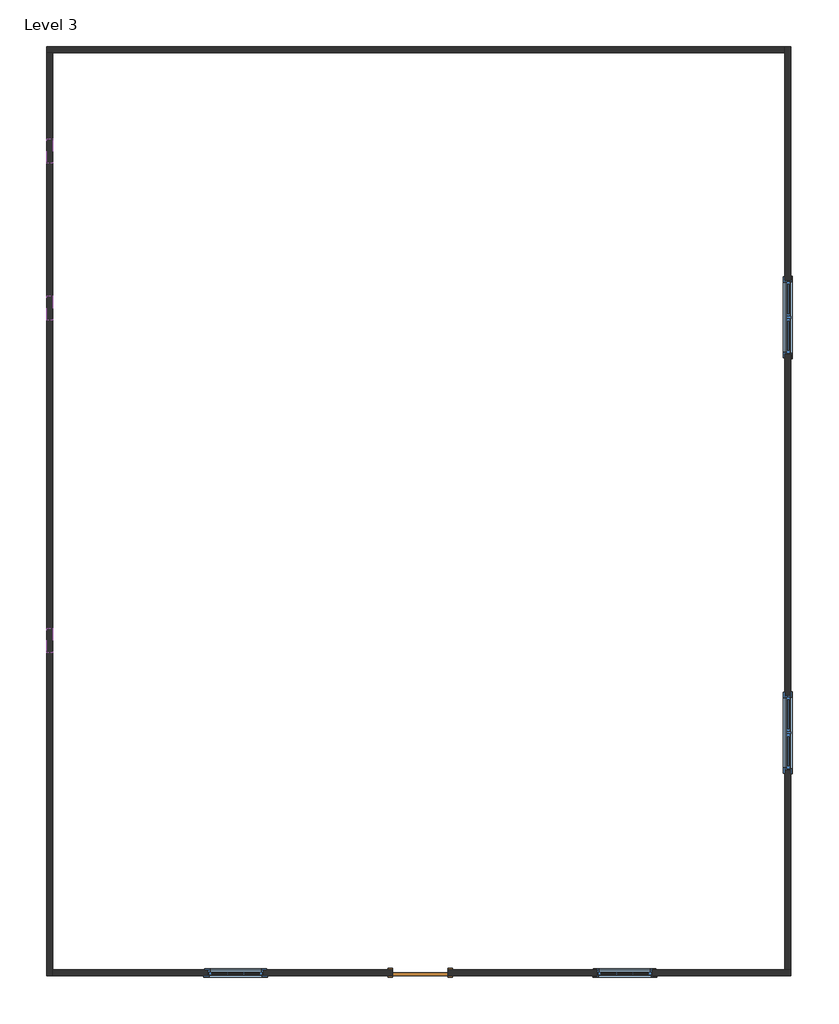
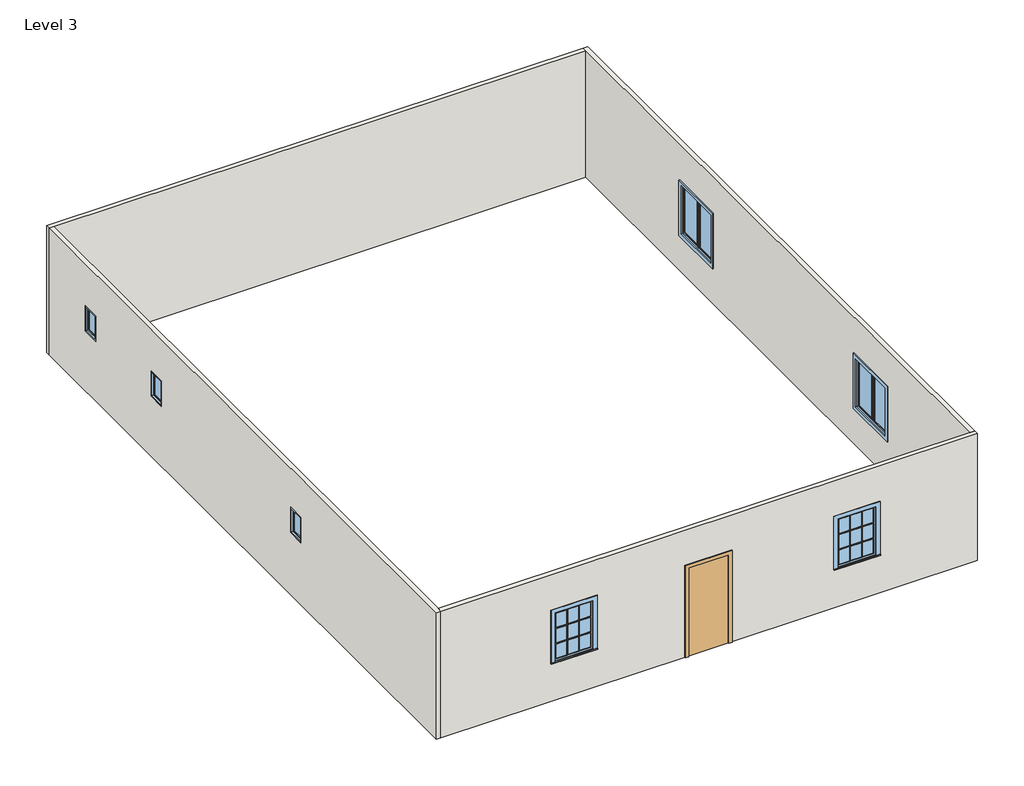
# One storey, incomplete: 7 windows, 4 walls, 1 door.
"""IFC4 building model written with IfcOpenShell, lengths in millimetres."""

from ifc_helpers import new_model, si_unit, origin, place, context, project, spatial, faceted_brep, transform, mapped, element, save
from components import door_048588e9, window_ad8769eb, window_90ef9153, window_a112695e

model = new_model("IFC4")

# Units and contexts
model_context = context("Model", 3, world=origin())
ifc_project = project(units=[si_unit("LENGTHUNIT", "METRE", prefix="MILLI")], contexts=[model_context])

# Site, building, storey
site = spatial("IfcSite", under=ifc_project)
building = spatial("IfcBuilding", under=site)
storey = spatial("IfcBuildingStorey", under=building, Name="Level 3", Elevation=3200.4)

# Door
placement = place(None, origin())
door_shape = door_048588e9(model_context)
element("IfcDoor", 1, ObjectType="Single-Flush : 36\" x 84\"", at=placement, inside=storey, context=model_context, shape_type="MappedRepresentation", body=[
    mapped(door_shape, transform((7865.9168112, -1990.8718204, 3200.4), x_axis=(-1.0, 0.0, 0.0), y_axis=(0.0, -1.0, 0.0), z_axis=(0.0, 0.0, 1.0))),
])

# Walls
element("IfcWall", 2, ObjectType="Generic - 4\" Brick", at=placement, inside=storey, context=model_context, shape_type="Brep", body=[
    faceted_brep([(1693.7168112, 13198.3281796, 3200.4), (1795.3168112, 13198.3281796, 3200.4), (13885.7168112, 13198.3281796, 3200.4), (13885.7168112, 13198.3281796, 6248.4), (1795.3168112, 13198.3281796, 6248.4), (1693.7168112, 13198.3281796, 6248.4), (1693.7168112, 13299.9281796, 3200.4), (1693.7168112, 13299.9281796, 6248.4), (13885.7168112, 13299.9281796, 6248.4), (13885.7168112, 13299.9281796, 3200.4)], [[[0, 1, 2, 3, 4, 5]], [[6, 7, 8, 9]], [[2, 1, 0, 6, 9]], [[0, 5, 7, 6]], [[3, 2, 9, 8]], [[5, 4, 3, 8, 7]]]),
])
element("IfcWall", 3, ObjectType="Generic - 4\" Brick", at=placement, inside=storey, context=model_context, shape_type="Brep", body=[
    faceted_brep([(1795.3168112, -2041.6718204, 3200.4), (1795.3168112, -1940.0718204, 3200.4), (1795.3168112, 13198.3281796, 3200.4), (1795.3168112, 13198.3281796, 6248.4), (1795.3168112, -1940.0718204, 6248.4), (1795.3168112, -2041.6718204, 6248.4), (1795.3168112, 8778.7281796, 5251.7031181), (1795.3168112, 9185.1281796, 5251.7031181), (1795.3168112, 9185.1281796, 4642.1031181), (1795.3168112, 8778.7281796, 4642.1031181), (1795.3168112, 11369.5281796, 5244.8693959), (1795.3168112, 11775.9281796, 5244.8693959), (1795.3168112, 11775.9281796, 4635.2693959), (1795.3168112, 11369.5281796, 4635.2693959), (1795.3168112, 3292.3281796, 5302.8886462), (1795.3168112, 3698.7281796, 5302.8886462), (1795.3168112, 3698.7281796, 4693.2886462), (1795.3168112, 3292.3281796, 4693.2886462), (1693.7168112, -2041.6718204, 3200.4), (1693.7168112, -2041.6718204, 6248.4), (1693.7168112, 13198.3281796, 6248.4), (1693.7168112, 13198.3281796, 3200.4), (1693.7168112, 8778.7281796, 5251.7031181), (1693.7168112, 8778.7281796, 4642.1031181), (1693.7168112, 9185.1281796, 4642.1031181), (1693.7168112, 9185.1281796, 5251.7031181), (1693.7168112, 11369.5281796, 5244.8693959), (1693.7168112, 11369.5281796, 4635.2693959), (1693.7168112, 11775.9281796, 4635.2693959), (1693.7168112, 11775.9281796, 5244.8693959), (1693.7168112, 3292.3281796, 5302.8886462), (1693.7168112, 3292.3281796, 4693.2886462), (1693.7168112, 3698.7281796, 4693.2886462), (1693.7168112, 3698.7281796, 5302.8886462)], [[[0, 1, 2, 3, 4, 5], [6, 7, 8, 9], [10, 11, 12, 13], [14, 15, 16, 17]], [[18, 19, 20, 21], [22, 23, 24, 25], [26, 27, 28, 29], [30, 31, 32, 33]], [[2, 1, 0, 18, 21]], [[0, 5, 19, 18]], [[3, 2, 21, 20]], [[5, 4, 3, 20, 19]], [[23, 22, 6, 9]], [[24, 23, 9, 8]], [[25, 24, 8, 7]], [[22, 25, 7, 6]], [[27, 26, 10, 13]], [[28, 27, 13, 12]], [[29, 28, 12, 11]], [[26, 29, 11, 10]], [[31, 30, 14, 17]], [[32, 31, 17, 16]], [[33, 32, 16, 15]], [[30, 33, 15, 14]]]),
])
element("IfcWall", 4, ObjectType="Generic - 4\" Brick", at=placement, inside=storey, context=model_context, shape_type="Brep", body=[
    faceted_brep([(7408.7168112, -1940.0718204, 5334.0), (7408.7168112, -1940.0718204, 3200.4), (1795.3168112, -1940.0718204, 3200.4), (1795.3168112, -1940.0718204, 6248.4), (13885.7168112, -1940.0718204, 6248.4), (13987.3168112, -1940.0718204, 6248.4), (13987.3168112, -1940.0718204, 3200.4), (13885.7168112, -1940.0718204, 3200.4), (8323.1168112, -1940.0718204, 3200.4), (8323.1168112, -1940.0718204, 5334.0), (4360.7168112, -1940.0718204, 5326.8905427), (4360.7168112, -1940.0718204, 4107.6905427), (5275.1168112, -1940.0718204, 4107.6905427), (5275.1168112, -1940.0718204, 5326.8905427), (10786.9168112, -1940.0718204, 5334.0), (10786.9168112, -1940.0718204, 4114.8), (11701.3168112, -1940.0718204, 4114.8), (11701.3168112, -1940.0718204, 5334.0), (1795.3168112, -2041.6718204, 3200.4), (7408.7168112, -2041.6718204, 3200.4), (7408.7168112, -2041.6718204, 5334.0), (8323.1168112, -2041.6718204, 5334.0), (8323.1168112, -2041.6718204, 3200.4), (13987.3168112, -2041.6718204, 3200.4), (13987.3168112, -2041.6718204, 6248.4), (1795.3168112, -2041.6718204, 6248.4), (4360.7168112, -2041.6718204, 5326.8905427), (5275.1168112, -2041.6718204, 5326.8905427), (5275.1168112, -2041.6718204, 4107.6905427), (4360.7168112, -2041.6718204, 4107.6905427), (10786.9168112, -2041.6718204, 5334.0), (11701.3168112, -2041.6718204, 5334.0), (11701.3168112, -2041.6718204, 4114.8), (10786.9168112, -2041.6718204, 4114.8)], [[[0, 1, 2, 3, 4, 5, 6, 7, 8, 9], [10, 11, 12, 13], [14, 15, 16, 17]], [[18, 19, 20, 21, 22, 23, 24, 25], [26, 27, 28, 29], [30, 31, 32, 33]], [[2, 1, 19, 18]], [[8, 7, 6, 23, 22]], [[6, 5, 24, 23]], [[3, 2, 18, 25]], [[5, 4, 3, 25, 24]], [[20, 19, 1, 0]], [[21, 20, 0, 9]], [[22, 21, 9, 8]], [[11, 10, 26, 29]], [[12, 11, 29, 28]], [[13, 12, 28, 27]], [[10, 13, 27, 26]], [[15, 14, 30, 33]], [[16, 15, 33, 32]], [[17, 16, 32, 31]], [[14, 17, 31, 30]]]),
])
element("IfcWall", 5, ObjectType="Generic - 4\" Brick", at=placement, inside=storey, context=model_context, shape_type="Brep", body=[
    faceted_brep([(13885.7168112, 13299.9281796, 3200.4), (13885.7168112, 13198.3281796, 3200.4), (13885.7168112, -1940.0718204, 3200.4), (13885.7168112, -1940.0718204, 6248.4), (13885.7168112, 13198.3281796, 6248.4), (13885.7168112, 13299.9281796, 6248.4), (13885.7168112, 1361.9281796, 5334.0), (13885.7168112, 1361.9281796, 4114.8), (13885.7168112, 2581.1281796, 4114.8), (13885.7168112, 2581.1281796, 5334.0), (13885.7168112, 8219.9281796, 5334.0), (13885.7168112, 8219.9281796, 4114.8), (13885.7168112, 9439.1281796, 4114.8), (13885.7168112, 9439.1281796, 5334.0), (13987.3168112, 13299.9281796, 3200.4), (13987.3168112, 13299.9281796, 6248.4), (13987.3168112, -1940.0718204, 6248.4), (13987.3168112, -1940.0718204, 3200.4), (13987.3168112, 1361.9281796, 5334.0), (13987.3168112, 2581.1281796, 5334.0), (13987.3168112, 2581.1281796, 4114.8), (13987.3168112, 1361.9281796, 4114.8), (13987.3168112, 8219.9281796, 5334.0), (13987.3168112, 9439.1281796, 5334.0), (13987.3168112, 9439.1281796, 4114.8), (13987.3168112, 8219.9281796, 4114.8)], [[[0, 1, 2, 3, 4, 5], [6, 7, 8, 9], [10, 11, 12, 13]], [[14, 15, 16, 17], [18, 19, 20, 21], [22, 23, 24, 25]], [[2, 1, 0, 14, 17]], [[0, 5, 15, 14]], [[3, 2, 17, 16]], [[5, 4, 3, 16, 15]], [[7, 6, 18, 21]], [[8, 7, 21, 20]], [[9, 8, 20, 19]], [[6, 9, 19, 18]], [[11, 10, 22, 25]], [[12, 11, 25, 24]], [[13, 12, 24, 23]], [[10, 13, 23, 22]]]),
])

# Windows
window_shape = window_ad8769eb(model_context)
element("IfcWindow", 6, ObjectType="Casement 3x3 with Trim : 36\" x 48\"", at=placement, inside=storey, context=model_context, shape_type="MappedRepresentation", body=[
    mapped(window_shape, transform((4817.9168112, -1990.8718204, 3193.2905427), x_axis=(-1.0, 0.0, 0.0), y_axis=(0.0, -1.0, 0.0), z_axis=(0.0, 0.0, 1.0))),
])
element("IfcWindow", 7, ObjectType="Casement 3x3 with Trim : 36\" x 48\"", at=placement, inside=storey, context=model_context, shape_type="MappedRepresentation", body=[
    mapped(window_shape, transform((11244.1168112, -1990.8718204, 3200.4), x_axis=(-1.0, 0.0, 0.0), y_axis=(0.0, -1.0, 0.0), z_axis=(0.0, 0.0, 1.0))),
])
window_2_shape = window_90ef9153(model_context)
element("IfcWindow", 8, ObjectType="Casement Dbl with Trim : 48\" x 48\"", at=placement, inside=storey, context=model_context, shape_type="MappedRepresentation", body=[
    mapped(window_2_shape, transform((13917.4668112, 1971.5281796, 3200.4), x_axis=(0.0, -1.0, 0.0), y_axis=(1.0, 0.0, 0.0), z_axis=(0.0, 0.0, 1.0))),
])
element("IfcWindow", 9, ObjectType="Casement Dbl with Trim : 48\" x 48\"", at=placement, inside=storey, context=model_context, shape_type="MappedRepresentation", body=[
    mapped(window_2_shape, transform((13917.4668112, 8829.5281796, 3200.4), x_axis=(0.0, -1.0, 0.0), y_axis=(1.0, 0.0, 0.0), z_axis=(0.0, 0.0, 1.0))),
])
window_3_shape = window_a112695e(model_context)
element("IfcWindow", 10, ObjectType="Fixed : 16\" x 24\"", at=placement, inside=storey, context=model_context, shape_type="MappedRepresentation", body=[
    mapped(window_3_shape, transform((1744.5168112, 8943.8281796, 3727.7031181), x_axis=(0.0, -1.0, 0.0), y_axis=(1.0, 0.0, 0.0), z_axis=(0.0, 0.0, 1.0))),
])
element("IfcWindow", 11, ObjectType="Fixed : 16\" x 24\"", at=placement, inside=storey, context=model_context, shape_type="MappedRepresentation", body=[
    mapped(window_3_shape, transform((1744.5168112, 11534.6281796, 3720.8693959), x_axis=(0.0, -1.0, 0.0), y_axis=(1.0, 0.0, 0.0), z_axis=(0.0, 0.0, 1.0))),
])
element("IfcWindow", 12, ObjectType="Fixed : 16\" x 24\"", at=placement, inside=storey, context=model_context, shape_type="MappedRepresentation", body=[
    mapped(window_3_shape, transform((1744.5168112, 3457.4281796, 3778.8886462), x_axis=(0.0, -1.0, 0.0), y_axis=(1.0, 0.0, 0.0), z_axis=(0.0, 0.0, 1.0))),
])

save(model, "model.ifc")

# Revit data of these elements
# Type "Single-Flush : 36\" x 84\""
#   Type Mark = "1"
#   Construction Type Id = "MDOOR"
#   Assembly Code = "C1020"
#   Analytic Construction = "Metal"
#   Thickness = 0' - 2"
#   Heat Transfer Coefficient (U) = 0.651978 BTU/(h·ft²·°F)
#   Height = 7' - 0"
#   Trim Projection Ext = 0' - 1"
#   Trim Projection Int = 0' - 1"
#   Trim Width = 0' - 3"
#   Width = 3' - 0"
#   Define Thermal Properties by = 1
#   Door Material = Door - Panel
#   Frame Material = Door - Frame
#   Visual Light Transmittance = 0
#   Solar Heat Gain Coefficient = 0
#   Function = (empty or 0)
#   Wall Closure = (empty or 0)
# Type "Generic - 4\" Brick"
#   Assembly Code = "B2010"
#   Layers, outside or top first: 0' - 4" "Brick, Common" (function 1)
# Type "Casement 3x3 with Trim : 36\" x 48\""
#   Type Mark = "10"
#   Construction Type Id = "GSP4R"
#   Assembly Code = "B2020100"
#   Analytic Construction = "1/8 in Pilkington single glazing"
#   Visual Light Transmittance = 0.9
#   Solar Heat Gain Coefficient = 0.78
#   Heat Transfer Coefficient (U) = 0.6496 BTU/(h·ft²·°F)
#   Height = 4' - 0"
#   Default Sill Height = 3' - 0"
#   Trim Projection - Ext. = 0' - 0 1/2"
#   Trim Projection - Int. = 0' - 0 3/4"
#   Trim Width - Exterior = 0' - 3 1/2"
#   Trim Width - Interior = 0' - 3 1/2"
#   Width = 3' - 0"
#   Window Inset = 0' - 0 3/4"
#   Define Thermal Properties by = 1
#   Glass Pane Material = Glass
#   Sash Material = Sash
#   Trim Exterior Material = Trim
#   Trim Interior Material = Trim
#   Wall Closure = (empty or 0)
# Type "Casement Dbl with Trim : 48\" x 48\""
#   Type Mark = "13"
#   Construction Type Id = "GSP4R"
#   Assembly Code = "B2020100"
#   Analytic Construction = "1/8 in Pilkington single glazing"
#   Visual Light Transmittance = 0.9
#   Solar Heat Gain Coefficient = 0.78
#   Heat Transfer Coefficient (U) = 0.6496 BTU/(h·ft²·°F)
#   Height = 4' - 0"
#   Default Sill Height = 3' - 0"
#   Trim Projection - Ext. = 0' - 0 1/2"
#   Trim Projection - Int. = 0' - 0 3/4"
#   Trim Width - Exterior = 0' - 3 1/2"
#   Trim Width - Interior = 0' - 3 1/2"
#   Width = 4' - 0"
#   Window Inset = 0' - 0 3/4"
#   Define Thermal Properties by = 1
#   Glass Pane Material = Glass
#   Sash Material = Sash
#   Trim Exterior Material = Trim
#   Trim Interior Material = Trim
#   Wall Closure = (empty or 0)
# Type "Fixed : 16\" x 24\""
#   Type Mark = "4"
#   Construction Type Id = "GSP4R"
#   Assembly Code = "B2020100"
#   Analytic Construction = "1/8 in Pilkington single glazing"
#   Visual Light Transmittance = 0.9
#   Solar Heat Gain Coefficient = 0.78
#   Heat Transfer Coefficient (U) = 0.6496 BTU/(h·ft²·°F)
#   Height = 2' - 0"
#   Default Sill Height = 3' - 0"
#   Width = 1' - 4"
#   Window Inset = 0' - 0 3/4"
#   Define Thermal Properties by = 1
#   Glass Pane Material = Glass
#   Sash Material = Sash
#   Wall Closure = (empty or 0)
# Element 1 (IfcDoor, "Single-Flush : 36\" x 84\"")
#   Phase Created = New Construction
#   Materials on its faces: "Door - Frame", "Door - Panel"
# Elements 2, 3, 4, 5 (IfcWall, "Generic - 4\" Brick")
#   Top Offset = 0' - 0"
#   Base Offset = 0' - 0"
#   Unconnected Height = 10' - 0"
#   wall height = 10' - 0"
#   Phase Created = New Construction
#   Base Constraint = Level 3
#   Materials on its faces: "Brick, Common"
# Element 6 (IfcWindow, "Casement 3x3 with Trim : 36\" x 48\"")
#   Mark = "15"
#   Phase Created = New Construction
#   Materials on its faces: "Sash", "Glass", "Trim"
# Element 7 (IfcWindow, "Casement 3x3 with Trim : 36\" x 48\"")
#   Mark = "16"
#   Phase Created = New Construction
#   Materials on its faces: "Sash", "Glass", "Trim"
# Element 8 (IfcWindow, "Casement Dbl with Trim : 48\" x 48\"")
#   Mark = "27"
#   Phase Created = New Construction
#   Materials on its faces: "Sash", "Trim", "Glass"
# Element 9 (IfcWindow, "Casement Dbl with Trim : 48\" x 48\"")
#   Mark = "29"
#   Phase Created = New Construction
#   Materials on its faces: "Sash", "Trim", "Glass"
# Element 10 (IfcWindow, "Fixed : 16\" x 24\"")
#   Mark = "3"
#   Phase Created = New Construction
#   Materials on its faces: "Sash", "Glass"
# Element 11 (IfcWindow, "Fixed : 16\" x 24\"")
#   Mark = "4"
#   Phase Created = New Construction
#   Materials on its faces: "Sash", "Glass"
# Element 12 (IfcWindow, "Fixed : 16\" x 24\"")
#   Mark = "9"
#   Phase Created = New Construction
#   Materials on its faces: "Sash", "Glass"
# Materials
#   "Door - Panel": class "Wood", colour RGB 210 159 95, transparency 0
#   "Door - Frame": colour RGB 118 70 51, transparency 0
#   "Brick, Common": class "Masonry", colour RGB 170 98 104, transparency 0, Description = "Common brick", Cost = 0
#   "Glass": class "Glass", colour RGB 0 128 192, transparency 0.75, Description = "Soda Lime Glass", Cost = 0
#   "Sash": class "Wood", colour RGB 224 178 126, transparency 0
#   "Trim": class "Wood", colour RGB 224 178 126, transparency 0
